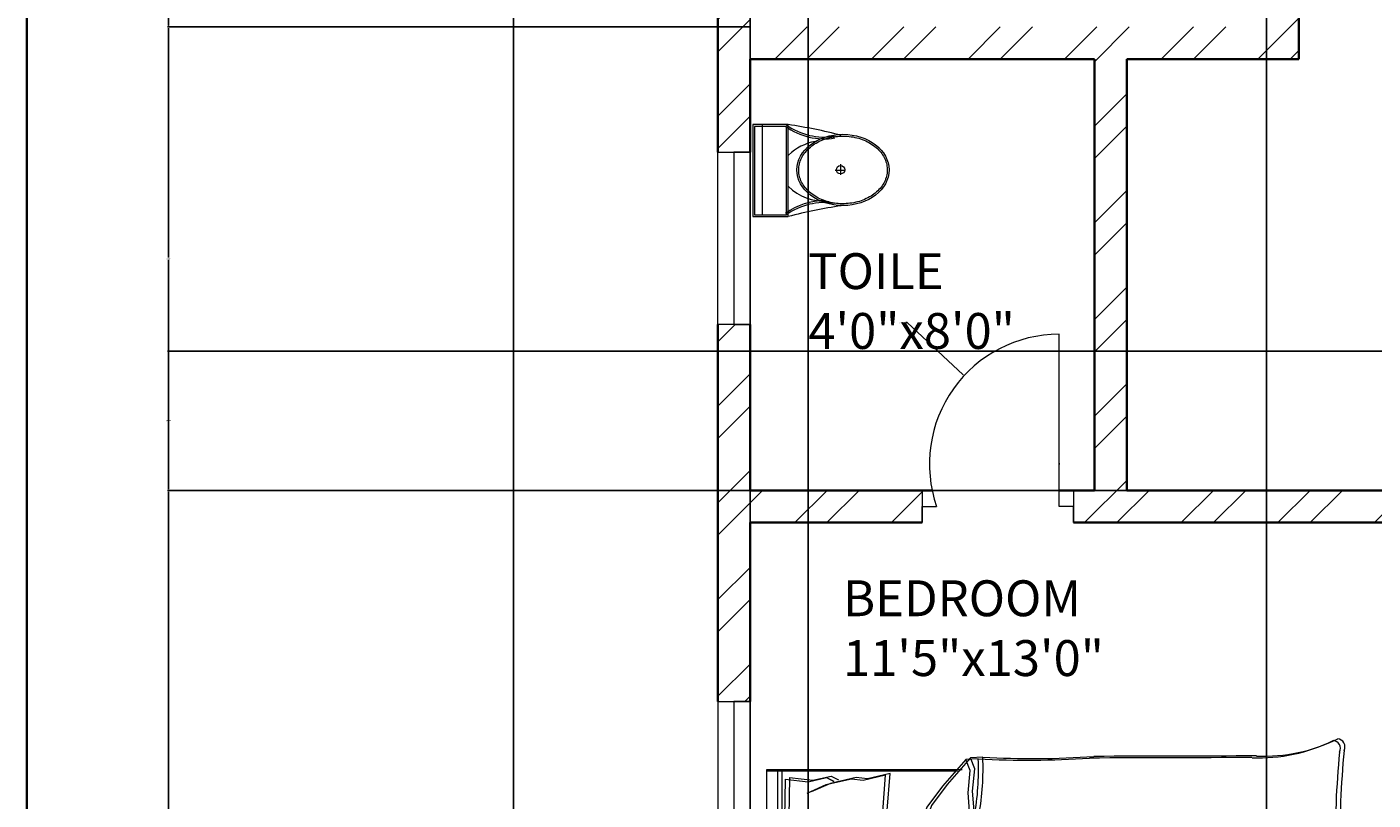
# Model space of a CAD drawing. Units: inches. Extents: x 2008 to 2657, y 1077 to 2165.
# Tile 2 of 16: x 2008 to 2196, y 1309 to 1417. Entities that reach past the tile are written whole.
import ezdxf

# ---------------------------------------------------------------- set-up
doc = ezdxf.new("R2010")
doc.units = ezdxf.units.IN
for name, color, linetype, lineweight in [('A-ANNO-DIMS', 2, 'Continuous', 18), ('A-ANNO-TTLB', 7, 'Continuous', 35), ('A-AREA-IDEN', 4, 'Continuous', 18), ('A-DOOR', 11, 'Continuous', 18), ('A-FLOR-FIXT', 8, 'Continuous', 18), ('A-FURN', 8, 'Continuous', 13), ('A-GLAZ', 191, 'Continuous', 18), ('A-WALL', 7, 'Continuous', 35)]:
    doc.layers.add(name, color=color, linetype=linetype, lineweight=lineweight)
doc.layers.add('A-WALL-PATT', color=30, linetype='Continuous', lineweight=13, true_color=0xf8991e)
doc.styles.get("Standard").update_dxf_attribs({"font": 'arial.ttf'})
doc.dimstyles.get("Standard").update_dxf_attribs({"dimtxt": 0.18, "dimasz": 0.18, "dimexe": 0.18, "dimexo": 0.0625, "dimgap": 0.09, "dimtad": 0, "dimtih": 1, "dimtoh": 1, "dimdec": 4, "dimzin": 0, "dimdsep": 46, "dimtxsty": 'Standard', "dimcen": 0.09, "dimadec": 0, "dimazin": 0, "dimtfac": 1, "dimtdec": 4, "dimtofl": 0, "dimtmove": 0, "dimatfit": 3, "dimfxl": 1, "dimtolj": 1, "dimtzin": 0, "dimarcsym": 0})

# ---------------------------------------------------------------- blocks, each defined once
blk = doc.blocks.new('A$C31115884')
for p, q in [((283.1, 497.7), (223.4, 497.7)), ((257.5, 466.4), (257.5, 523.2)), ((0, 200), (0, 0)), ((520, 200), (0, 200)), ((10, 190), (10, 10)), ((510, 190), (10, 190)), ((510, 10), (510, 190)), ((520, 0), (520, 200)), ((510, 54.5), (0, 54.5)), ((10, 10), (510, 10)), ((0, 0), (520, 0))]:
    blk.add_line(p, q)
blk.add_circle((255.6, 496.4), 23.6)
for centre, radius, start, end in [((2777.7, -204.6), 2807, 165.4549, 171.71327), ((-294.5, 403.3), 364.7, 324.20913, 9.34987), ((-294.5, 403.3), 374.7, 324.20913, 9.34987), ((805.8, 403.3), 364.7, 170.65013, 215.79087), ((3237, 905), 2807, 188.28673, 194.5451), ((139.5, 406.2), 293.5, 315.84364, 2.65635), ((805.8, 403.3), 374.7, 179.20365, 215.79087), ((383.6, 406.2), 293.5, 190.27735, 224.15636)]:
    blk.add_arc(centre, radius, start, end)
blk.add_ellipse((256.2, 509.9), major_axis=(0, -260.7), ratio=0.772727)
blk.add_open_spline([(256.2, 259.2), (263.1, 259.2), (270, 259.7), (287.8, 262.3), (298.7, 265.1), (319.9, 273.1), (330.2, 278.4), (350.1, 291.1), (359.7, 298.7), (377.7, 315.9), (386.2, 325.5), (401.7, 346.6), (408.8, 358.1), (421.3, 382.5), (426.8, 395.5), (435.9, 422.4), (439.5, 436.4), (444.8, 465.1), (446.5, 479.7), (447.9, 509.2), (447.6, 524), (445, 553.3), (442.7, 567.8), (436.3, 596), (432.1, 609.7), (421.9, 636), (416, 648.6), (402.5, 672.1), (395, 683), (378.6, 703), (369.8, 712.1), (351.1, 728), (341.3, 734.8), (320.9, 746.2), (310.4, 750.7), (288.9, 757.3), (278, 759.4), (256, 761), (245, 760.6), (223.1, 757.2), (212.3, 754.3), (191.1, 746.1), (180.8, 740.7), (160.9, 727.8), (151.4, 720.1), (133.5, 702.7), (125.1, 693), (109.6, 671.7), (102.6, 660.2), (90.2, 635.7), (84.9, 622.7), (76, 595.6), (72.4, 581.6), (67.2, 552.9), (65.6, 538.2), (64.4, 508.8), (64.8, 494), (67.5, 464.7), (69.9, 450.2), (76.6, 422), (80.8, 408.3), (91.1, 382.2), (97.2, 369.7), (110.8, 346.3), (118.4, 335.4), (134.8, 315.6), (143.7, 306.7), (162.4, 290.9), (172.3, 284.2), (192.8, 273), (203.3, 268.6), (224.8, 262.2), (235.8, 260.2), (249.9, 259.3), (253, 259.2), (256.2, 259.2)], degree=3, knots=[0, 0, 0, 0, 0.110105, 0.110105, 0.285049, 0.285049, 0.459994, 0.459994, 0.634938, 0.634938, 0.809882, 0.809882, 0.984827, 0.984827, 1.159771, 1.159771, 1.334715, 1.334715, 1.50966, 1.50966, 1.684604, 1.684604, 1.859549, 1.859549, 2.034493, 2.034493, 2.209437, 2.209437, 2.384382, 2.384382, 2.559326, 2.559326, 2.73427, 2.73427, 2.909215, 2.909215, 3.084159, 3.084159, 3.259103, 3.259103, 3.434048, 3.434048, 3.608992, 3.608992, 3.783936, 3.783936, 3.958881, 3.958881, 4.133825, 4.133825, 4.30877, 4.30877, 4.483714, 4.483714, 4.658658, 4.658658, 4.833603, 4.833603, 5.008547, 5.008547, 5.183491, 5.183491, 5.358436, 5.358436, 5.53338, 5.53338, 5.708324, 5.708324, 5.883269, 5.883269, 6.058213, 6.058213, 6.233158, 6.233158, 6.283185, 6.283185, 6.283185, 6.283185])
blk = doc.blocks.new('BED-DOUBLE')
for p, q in [((27.75, 52.87), (24.5, 49.16)), ((27.75, 52.87), (24.5, 49.16)), ((28.39, 53.1), (25.14, 49.39)), ((28.39, 53.1), (25.14, 49.39)), ((29.49, 52.95), (27.75, 52.87, 3.87)), ((29.49, 52.95), (27.75, 52.87, 3.87)), ((28.37, 51.33), (27.75, 52.87)), ((28.37, 51.33), (27.75, 52.87)), ((30.13, 53.18), (28.39, 53.1, 3.87)), ((30.13, 53.18), (28.39, 53.1, 3.87)), ((29, 51.56), (28.39, 53.1)), ((29, 51.56), (28.39, 53.1)), ((0, 51.49), (0.64, 51.49)), ((0, 3.48), (0, 51.49)), ((0, 51.27), (26.61, 51.27)), ((0, 51.27), (26.61, 51.27)), ((0.64, 51.49), (27.25, 51.49)), ((0.64, 51.49), (27.25, 51.49)), ((1.53, 3.48), (1.53, 51.27)), ((1.53, 3.48), (1.53, 51.27)), ((2.17, 3.7), (2.17, 51.49)), ((2.17, 3.7), (2.17, 51.49)), ((16.57, 50.7), (13.43, 49.92)), ((16.57, 50.7), (13.43, 49.92)), ((17.21, 50.93), (14.07, 50.15)), ((17.21, 50.93), (14.07, 50.15)), ((16.17, 45.57), (16.57, 50.7)), ((16.17, 45.57), (16.57, 50.7)), ((16.81, 45.8), (17.21, 50.93)), ((16.81, 45.8), (17.21, 50.93)), ((28.06, 48.23), (28.37, 51.33)), ((28.06, 48.23), (28.37, 51.33)), ((28.7, 48.46), (29, 51.56)), ((28.7, 48.46), (29, 51.56)), ((2.56, 50.11), (2.46, 44.71)), ((2.56, 50.11), (2.46, 44.71)), ((2.56, 50.11), (5.77, 49.73)), ((2.56, 50.11), (5.77, 49.73)), ((3.2, 50.34), (3.1, 44.94)), ((3.2, 50.34), (3.1, 44.94)), ((3.2, 50.34), (6.41, 49.96)), ((3.2, 50.34), (6.41, 49.96)), ((8.26, 49.31), (5.58, 48.13)), ((8.26, 49.31), (5.58, 48.13)), ((5.77, 49.73), (8.34, 50.33)), ((5.77, 49.73), (8.34, 50.33)), ((8.9, 49.54), (6.22, 48.36)), ((8.9, 49.54), (6.22, 48.36)), ((6.41, 49.96), (8.98, 50.56)), ((6.41, 49.96), (8.98, 50.56)), ((11.83, 50.11), (8.26, 49.31)), ((11.83, 50.11), (8.26, 49.31)), ((8.34, 50.33), (9.38, 49.82)), ((8.34, 50.33), (9.38, 49.81)), ((12.47, 50.34), (8.9, 49.54)), ((12.47, 50.34), (8.9, 49.54)), ((8.98, 50.56), (10.02, 50.04)), ((8.98, 50.56), (10.02, 50.04)), ((13.43, 49.92), (11.83, 50.11)), ((13.43, 49.92), (11.83, 50.11)), ((14.07, 50.15), (12.47, 50.34)), ((14.07, 50.15), (12.47, 50.34)), ((24.5, 49.16), (22.33, 46.22)), ((24.5, 49.16), (22.33, 46.22)), ((25.14, 49.39), (22.97, 46.45)), ((25.14, 49.39), (22.97, 46.45)), ((28.37, 44.36), (28.06, 48.23)), ((28.37, 44.36), (28.06, 48.23)), ((29, 44.59), (28.7, 48.46)), ((29, 44.59), (28.7, 48.46)), ((2.46, 44.71), (2.54, 45.71)), ((2.46, 44.71), (2.54, 45.71)), ((2.54, 45.71), (3.07, 41.91)), ((2.54, 45.71), (3.07, 41.91)), ((3.1, 44.94), (3.18, 45.94)), ((3.1, 44.94), (3.18, 45.94)), ((3.18, 45.94), (3.71, 42.14)), ((3.18, 45.94), (3.71, 42.14)), ((16.73, 43.61), (16.17, 45.57)), ((16.73, 43.61), (16.17, 45.57)), ((17.37, 43.84), (16.81, 45.8)), ((17.37, 43.83), (16.81, 45.8)), ((22.33, 46.22), (20.32, 40.64)), ((22.33, 46.22), (20.32, 40.64)), ((22.97, 46.45), (20.96, 40.87)), ((22.97, 46.45), (20.96, 40.87)), ((16.3, 36.6), (16.73, 43.61)), ((16.3, 36.6), (16.73, 43.61)), ((16.93, 36.83), (17.37, 43.84)), ((16.93, 36.82), (17.37, 43.83)), ((28.83, 40.95), (28.37, 44.36)), ((28.83, 40.95), (28.37, 44.36)), ((29.47, 41.18), (29, 44.59)), ((29.47, 41.18), (29, 44.59)), ((3.07, 41.91), (4.42, 36.5)), ((3.07, 41.91), (4.42, 36.5)), ((3.71, 42.14), (5.06, 36.72)), ((3.71, 42.14), (5.06, 36.72)), ((4.31, 39.43), (3.72, 37.36)), ((4.31, 39.43), (3.72, 37.36)), ((20.32, 40.64), (17.38, 32.31)), ((20.32, 40.64), (17.38, 32.31)), ((20.96, 40.87), (18.02, 32.54)), ((20.96, 40.87), (18.02, 32.53)), ((29.76, 38.94), (28.83, 40.95)), ((29.76, 38.94), (28.83, 40.95)), ((30.4, 39.17), (29.47, 41.18)), ((30.4, 39.17), (29.47, 41.18)), ((79.25, 15.06), (79.25, 39.68)), ((79.25, 15.06), (79.25, 39.68)), ((79.88, 15.29), (79.88, 39.91)), ((79.88, 15.29), (79.88, 39.91)), ((3.67, 39.2), (3.08, 37.14)), ((3.67, 39.2), (3.08, 37.14)), ((30.38, 36.46), (29.76, 38.94)), ((30.38, 36.46), (29.76, 38.94)), ((31.02, 36.69), (30.4, 39.17)), ((31.02, 36.69), (30.4, 39.17)), ((3.08, 37.14), (2.54, 34.21)), ((3.08, 37.14), (2.54, 34.2)), ((3.72, 37.36), (3.18, 34.43)), ((3.72, 37.36), (3.18, 34.43)), ((15.63, 32.56), (16.3, 36.6)), ((15.63, 32.56), (16.3, 36.6)), ((16.27, 32.79), (16.93, 36.83)), ((16.27, 32.79), (16.93, 36.82)), ((23.88, 34.45), (28.37, 36.15)), ((23.88, 34.45), (28.37, 36.15)), ((24.52, 34.68), (29, 36.38)), ((24.52, 34.68), (29, 36.38)), ((28.37, 36.15), (30.38, 36.46)), ((28.37, 36.15), (30.38, 36.46)), ((29, 36.38), (31.02, 36.69)), ((29, 36.38), (31.02, 36.69)), ((2.54, 34.21), (2.56, 33.88)), ((2.54, 34.2), (2.56, 33.88)), ((2.56, 33.88), (2.98, 29.46)), ((2.56, 33.88), (2.98, 29.46)), ((3.18, 34.43), (3.2, 34.11)), ((3.18, 34.43), (3.2, 34.11)), ((3.2, 34.11), (3.62, 29.68)), ((3.2, 34.11), (3.62, 29.68)), ((16.74, 30.75), (15.45, 33.82)), ((16.74, 30.75), (15.45, 33.82)), ((17.38, 30.98), (16.09, 34.05)), ((17.38, 30.98), (16.09, 34.05)), ((17.38, 30.26), (23.88, 34.45)), ((17.38, 30.26), (23.88, 34.45)), ((18.02, 30.49), (24.52, 34.68)), ((18.02, 30.49), (24.52, 34.68)), ((16.89, 28.3), (16.74, 30.75)), ((16.89, 28.3), (16.74, 30.75)), ((17.53, 28.53), (17.38, 30.98)), ((17.53, 28.53), (17.38, 30.98)), ((2.98, 29.46), (2.49, 27.98)), ((2.98, 29.46), (2.49, 27.98)), ((3.62, 29.68), (3.13, 28.21)), ((3.62, 29.68), (3.13, 28.21)), ((3.13, 28.21), (8.51, 27.96)), ((3.13, 28.21), (8.51, 27.96)), ((13.02, 27.66), (14.86, 28.36)), ((13.02, 27.66), (14.86, 28.36)), ((14.22, 28.13), (16.89, 28.3)), ((14.22, 28.13), (16.89, 28.3)), ((14.86, 28.36), (17.53, 28.53)), ((14.86, 28.36), (17.53, 28.53)), ((1.87, 25.98), (7.22, 26.56)), ((1.87, 25.98), (7.22, 26.56)), ((2.49, 27.98), (7.87, 27.73)), ((2.49, 27.98), (7.87, 27.73)), ((2.51, 26.21), (7.86, 26.79)), ((2.51, 26.21), (7.86, 26.79)), ((7.22, 26.56), (10.4, 27.14)), ((7.22, 26.56), (10.4, 27.14)), ((7.86, 26.79), (11.04, 27.37)), ((7.86, 26.79), (11.04, 27.37)), ((7.87, 27.73), (11.08, 27.36)), ((7.87, 27.73), (11.08, 27.36)), ((8.51, 27.96), (11.72, 27.58)), ((8.51, 27.96), (11.72, 27.58)), ((10.4, 27.14), (11.7, 27.14)), ((10.4, 27.14), (11.7, 27.14)), ((11.04, 27.37), (12.34, 27.37)), ((11.04, 27.37), (12.34, 27.37)), ((11.08, 27.36), (12.38, 27.44)), ((11.08, 27.36), (12.38, 27.44)), ((11.7, 27.14), (13.58, 26.56)), ((11.7, 27.14), (13.58, 26.56)), ((11.72, 27.58), (13.02, 27.66)), ((11.72, 27.58), (13.02, 27.66)), ((12.34, 27.37), (14.22, 26.79)), ((12.34, 27.37), (14.22, 26.79)), ((12.38, 27.44), (14.22, 28.13)), ((12.38, 27.44), (14.22, 28.13)), ((13.58, 26.56), (16.26, 26.56)), ((13.58, 26.56), (16.26, 26.56)), ((14.22, 26.79), (16.9, 26.79)), ((14.22, 26.79), (16.9, 26.79)), ((16.26, 26.56), (16.26, 24.1)), ((16.26, 26.56), (16.26, 24.1)), ((16.9, 26.79), (16.9, 24.33)), ((16.9, 26.79), (16.9, 24.33)), ((2.45, 24.54), (1.87, 25.98)), ((2.45, 24.54), (1.87, 25.98)), ((2.3, 20.09), (2.45, 24.54)), ((2.3, 20.09), (2.45, 24.54)), ((3.09, 24.77), (2.51, 26.21)), ((3.09, 24.77), (2.51, 26.21)), ((2.94, 20.32), (3.09, 24.77)), ((2.94, 20.32), (3.09, 24.77)), ((16.17, 19.38), (16.57, 24.52)), ((16.17, 19.38), (16.57, 24.52)), ((16.81, 19.61), (17.21, 24.74)), ((16.81, 19.61), (17.21, 24.74)), ((16.26, 24.1), (15.17, 20.96)), ((16.26, 24.1), (15.17, 20.96)), ((16.9, 24.33), (15.81, 21.19)), ((16.9, 24.33), (15.81, 21.19)), ((2.3, 19.77), (2.3, 20.09)), ((2.3, 19.77), (2.3, 20.09)), ((3.03, 16.88), (2.3, 19.77)), ((3.03, 16.88), (2.3, 19.77)), ((2.94, 20), (2.94, 20.32)), ((2.94, 20), (2.94, 20.32)), ((3.67, 17.11), (2.94, 20)), ((3.67, 17.11), (2.94, 20)), ((16.73, 17.42), (16.17, 19.38)), ((16.73, 17.42), (16.17, 19.38)), ((17.37, 17.65), (16.81, 19.61)), ((17.37, 17.65), (16.81, 19.61)), ((3.32, 12.11), (4.33, 17.6)), ((3.32, 12.11), (4.33, 17.6)), ((4.39, 15.08), (3.67, 17.11)), ((4.39, 15.08), (3.67, 17.11)), ((3.96, 12.34), (4.97, 17.83)), ((3.96, 12.34), (4.97, 17.83)), ((16.3, 10.41), (16.73, 17.42)), ((16.3, 10.41), (16.73, 17.42)), ((16.93, 10.64), (17.37, 17.65)), ((16.93, 10.64), (17.37, 17.65)), ((3.75, 14.86), (3.03, 16.88)), ((3.75, 14.86), (3.03, 16.88)), ((3.03, 8.29), (3.32, 12.11)), ((3.03, 8.29), (3.32, 12.11)), ((3.67, 8.51), (3.96, 12.34)), ((3.67, 8.51), (3.96, 12.34)), ((15.63, 6.38), (16.3, 10.41)), ((15.63, 6.38), (16.3, 10.41)), ((16.27, 6.61), (16.93, 10.64)), ((16.27, 6.61), (16.93, 10.64)), ((16.3, 10.41), (16.62, 9.28)), ((16.3, 10.41), (16.62, 9.28)), ((16.93, 10.64), (17.26, 9.51)), ((16.93, 10.64), (17.26, 9.51)), ((17.26, 9.51), (17.98, 4.41)), ((17.26, 9.51), (17.98, 4.41)), ((3.01, 8.18), (3.03, 8.29)), ((3.01, 8.18), (3.03, 8.29)), ((3.34, 3.9), (3.01, 8.18)), ((3.34, 3.9), (3.01, 8.18)), ((3.65, 8.41), (3.67, 8.51)), ((3.65, 8.41), (3.67, 8.51)), ((3.98, 4.13), (3.65, 8.41)), ((3.98, 4.13), (3.65, 8.41)), ((16.62, 9.28), (17.34, 4.18)), ((16.62, 9.28), (17.34, 4.18)), ((8.96, 5.05), (6.21, 6.06)), ((8.96, 5.05), (6.21, 6.06)), ((9.59, 5.28), (6.85, 6.29)), ((9.59, 5.28), (6.85, 6.29)), ((3.32, 3.9), (6.5, 4.47)), ((3.32, 3.89), (6.5, 4.47)), ((3.96, 4.12), (7.14, 4.7)), ((3.96, 4.12), (7.14, 4.7)), ((6.5, 4.47), (9.1, 4.04)), ((6.5, 4.47), (9.1, 4.04)), ((7.14, 4.7), (9.74, 4.27)), ((7.14, 4.7), (9.74, 4.27)), ((12.57, 4.47), (8.96, 5.05)), ((12.57, 4.47), (8.96, 5.05)), ((9.1, 4.04), (10.11, 4.62)), ((9.1, 4.04), (10.11, 4.62)), ((13.21, 4.7), (9.59, 5.28)), ((13.21, 4.7), (9.59, 5.28)), ((9.74, 4.27), (10.75, 4.85)), ((9.74, 4.27), (10.75, 4.85)), ((14.16, 4.76), (12.57, 4.47)), ((14.16, 4.76), (12.57, 4.47)), ((14.8, 4.99), (13.21, 4.7)), ((14.8, 4.99), (13.21, 4.7)), ((17.34, 4.18), (14.16, 4.76)), ((17.34, 4.18), (14.16, 4.76)), ((17.98, 4.41), (14.8, 4.99)), ((17.98, 4.41), (14.8, 4.99)), ((18.11, 3.48), (0, 3.48)), ((18.11, 3.48), (0, 3.48)), ((18.75, 3.7), (0.64, 3.7)), ((18.75, 3.7), (0.64, 3.7))]:
    blk.add_line(p, q)
for centre, radius, start, end in [((68.67, 76.16), 23.07, 267.4714, 296.4681), ((68.67, 76.16), 23.07, 267.4714, 296.4681), ((69.31, 76.39), 23.07, 267.4714, 296.4681), ((69.31, 76.39), 23.07, 267.4714, 296.4681), ((78.87, 54.41), 1.1, 332.6588, 86.02), ((78.87, 54.41), 1.1, 332.6588, 86.02), ((79.51, 54.64), 1.1, 332.6588, 86.02), ((79.51, 54.64), 1.1, 332.6588, 86.02), ((-6.66, 51.33), 36.18, 349.8763, 2.5657), ((-6.66, 51.33), 36.18, 349.8763, 2.5657), ((36.32, 182.27), 129.5, 266.9791, 273.8365), ((36.32, 182.27), 129.5, 266.9791, 273.8365), ((-6.02, 51.56), 36.18, 349.8763, 2.5657), ((-6.02, 51.56), 36.18, 349.8763, 2.5657), ((36.95, 182.49), 129.5, 266.9791, 273.8365), ((36.95, 182.49), 129.5, 266.9791, 273.8365), ((67.82, -4508.74), 4561.86, 90.00217, 90.28689), ((67.82, -4508.74), 4561.86, 90.00217, 90.28689), ((68.46, -4508.51), 4561.86, 90.00217, 90.28689), ((68.46, -4508.51), 4561.86, 90.00217, 90.28689), ((212.28, 41.15), 133.04, 174.4998, 180.6351), ((212.28, 41.15), 133.04, 174.4998, 180.6351), ((212.92, 41.38), 133.04, 174.4998, 180.6351), ((212.92, 41.38), 133.04, 174.4998, 180.6351), ((35.71, 43.97), 6.22, 168.6608, 203.7384), ((35.71, 43.97), 6.22, 168.6608, 203.7384), ((35.07, 43.74), 6.22, 168.6608, 203.7384), ((35.07, 43.74), 6.22, 168.6608, 203.7384), ((2.12, 31.38), 29.65, 10.6617, 19.8806), ((2.12, 31.38), 29.65, 10.6617, 19.8806), ((1.48, 31.15), 29.65, 10.6617, 19.8806), ((1.48, 31.15), 29.65, 10.6617, 19.8806), ((156.32, 17.76), 129.02, 171.7845, 186.9006), ((156.32, 17.76), 129.02, 171.7845, 186.9006), ((156.96, 17.98), 129.02, 171.7845, 186.9006), ((156.96, 17.98), 129.02, 171.7845, 186.9006), ((30.44, 36.64), 0.185, 250.2464, 1.1377), ((30.44, 36.64), 0.185, 250.2464, 1.1377), ((31.08, 36.87), 0.185, 250.2464, 1.1377), ((31.08, 36.86), 0.185, 250.2464, 1.1377), ((182.05, 21.36), 164.97, 176.0865, 186.7821), ((182.05, 21.36), 164.97, 176.0865, 186.7821), ((182.69, 21.59), 164.97, 176.0865, 186.7821), ((182.69, 21.59), 164.97, 176.0865, 186.7821), ((-23.71, -17.22), 106.46, 13.3832, 17.7053), ((-23.71, -17.22), 106.46, 13.3832, 17.7053), ((-23.07, -16.99), 106.46, 13.3832, 17.7053), ((-23.07, -16.99), 106.46, 13.3832, 17.7053), ((200.84, 21.43), 121.76, 182.9958, 189.4091), ((200.84, 21.43), 121.76, 182.9958, 189.4091), ((201.48, 21.66), 121.76, 182.9958, 189.4091), ((201.48, 21.66), 121.76, 182.9958, 189.4091), ((20.1, 85.16), 83.31, 268.7218, 275.604), ((20.1, 85.16), 83.31, 268.7218, 275.604), ((20.74, 85.39), 83.31, 268.7218, 275.604), ((20.74, 85.39), 83.31, 268.7218, 275.604), ((31.17, -167.31), 170.11, 88.4762, 91.0082), ((31.17, -167.31), 170.11, 88.4762, 91.0082), ((31.81, -167.08), 170.11, 88.4762, 91.0082), ((31.81, -167.08), 170.11, 88.4762, 91.0082), ((50.61, 484.82), 482.31, 268.2277, 271.7185), ((50.61, 484.82), 482.31, 268.2277, 271.7185), ((51.25, 485.05), 482.31, 268.2277, 271.7185), ((51.25, 485.05), 482.31, 268.2277, 271.7185), ((64.52, -26.9), 29.63, 76.0648, 88.9113), ((64.52, -26.9), 29.63, 76.0648, 88.9113), ((65.15, -26.67), 29.63, 76.0648, 88.9113), ((65.15, -26.67), 29.63, 76.0648, 88.9113), ((70.92, -21.43), 23.56, 67.9751, 86.652), ((70.92, -21.43), 23.56, 67.9751, 86.652), ((70.28, -21.66), 23.56, 67.9751, 86.652), ((70.28, -21.66), 23.56, 67.9751, 86.652), ((79.72, 1.09), 1.09, 236.1736, 23.4781), ((79.72, 1.09), 1.09, 236.1736, 23.4781), ((80.36, 1.32), 1.09, 236.1736, 23.4781), ((80.36, 1.32), 1.09, 236.1736, 23.4781)]:
    blk.add_arc(centre, radius, start, end)
blk = doc.blocks.new('WIN-24IN-A')
for p, q in [((0, 24), (4.5, 24)), ((0, 0), (0, 24)), ((4.5, 24), (2.25, 24)), ((2.25, 24), (2.25, 0)), ((4.5, 24), (4.5, 0)), ((4.5, 0), (0, 0)), ((2.25, 0), (4.5, 0))]:
    blk.add_line(p, q)
blk = doc.blocks.new('WIN-60IN-A')
for p, q in [((0, 60), (4.5, 60)), ((0, 60), (0, 0)), ((4.5, 60), (2.25, 60)), ((2.25, 60), (2.25, 0)), ((4.5, 0), (4.5, 60)), ((4.5, 0), (0, 0)), ((2.25, 0), (4.5, 0))]:
    blk.add_line(p, q)
blk = doc.blocks.new('*D31')
at = {"layer": 'A-ANNO-DIMS', "color": 0, "lineweight": -2, "transparency": 16777216}
for p, q in [((2076.26, 1562.18), (2076.26, 1140.44)), ((2576.76, 1188.61), (2576.76, 1140.44)), ((2076.44, 1140.62), (2326.12, 1140.62)), ((2576.58, 1140.62), (2326.91, 1140.62))]:
    blk.add_line(p, q, dxfattribs=at)
at = {"layer": 'A-ANNO-DIMS', "color": 0, "transparency": 16777216}
for points in [[(2076.44, 1140.65), (2076.44, 1140.59), (2076.26, 1140.62)], [(2576.58, 1140.65), (2576.58, 1140.59), (2576.76, 1140.62)]]:
    blk.add_solid(points, dxfattribs=at)
at = {"layer": 'Defpoints', "color": 0, "transparency": 16777216}
for p in [(2076.26, 1562.24), (2576.76, 1188.67), (2576.76, 1140.62)]:
    blk.add_point(p, dxfattribs=at)
at = {"layer": 'A-ANNO-DIMS', "color": 0, "transparency": 16777216, "insert": (2326.51, 1140.62), "char_height": 0.18, "attachment_point": 5}
blk.add_mtext('\\A1;500.5', dxfattribs=at)
blk = doc.blocks.new('*D39')
at = {"layer": 'A-ANNO-DIMS', "color": 0, "lineweight": -2, "transparency": 16777216}
for p, q in [((2109.2, 1352.17), (2028.03, 1352.17)), ((2028.21, 1351.99), (2028.21, 1290.11)), ((2028.21, 1227.85), (2028.21, 1289.74)), ((2109.2, 1227.67), (2028.03, 1227.67))]:
    blk.add_line(p, q, dxfattribs=at)
at = {"layer": 'A-ANNO-DIMS', "color": 0, "transparency": 16777216}
for points in [[(2028.18, 1351.99), (2028.24, 1351.99), (2028.21, 1352.17)], [(2028.18, 1227.85), (2028.24, 1227.85), (2028.21, 1227.67)]]:
    blk.add_solid(points, dxfattribs=at)
at = {"layer": 'Defpoints', "color": 0, "transparency": 16777216}
for p in [(2028.21, 1352.17), (2109.26, 1352.17), (2109.26, 1227.67)]:
    blk.add_point(p, dxfattribs=at)
at = {"layer": 'A-ANNO-DIMS', "color": 0, "transparency": 16777216, "insert": (2028.21, 1289.92), "char_height": 0.18, "attachment_point": 5}
blk.add_mtext('\\A1;124.5', dxfattribs=at)
blk = doc.blocks.new('*D40')
at = {"layer": 'A-ANNO-DIMS', "color": 0, "lineweight": -2, "transparency": 16777216}
for p, q in [((2109.2, 1416.74), (2028.03, 1416.74)), ((2028.21, 1416.56), (2028.21, 1384.64)), ((2028.21, 1352.35), (2028.21, 1384.28)), ((2109.2, 1352.17), (2028.03, 1352.17))]:
    blk.add_line(p, q, dxfattribs=at)
at = {"layer": 'A-ANNO-DIMS', "color": 0, "transparency": 16777216}
for points in [[(2028.18, 1416.56), (2028.24, 1416.56), (2028.21, 1416.74)], [(2028.18, 1352.35), (2028.24, 1352.35), (2028.21, 1352.17)]]:
    blk.add_solid(points, dxfattribs=at)
at = {"layer": 'Defpoints', "color": 0, "transparency": 16777216}
for p in [(2028.21, 1416.74), (2109.26, 1416.74), (2109.26, 1352.17)]:
    blk.add_point(p, dxfattribs=at)
at = {"layer": 'A-ANNO-DIMS', "color": 0, "transparency": 16777216, "insert": (2028.21, 1384.46), "char_height": 0.18, "attachment_point": 5}
blk.add_mtext('\\A1;64.57', dxfattribs=at)
blk = doc.blocks.new('*D41')
at = {"layer": 'A-ANNO-DIMS', "color": 0, "lineweight": -2, "transparency": 16777216}
for p, q in [((2109.2, 1514.24), (2028.03, 1514.24)), ((2028.21, 1514.06), (2028.21, 1465.67)), ((2028.21, 1416.92), (2028.21, 1465.31)), ((2109.2, 1416.74), (2028.03, 1416.74))]:
    blk.add_line(p, q, dxfattribs=at)
at = {"layer": 'A-ANNO-DIMS', "color": 0, "transparency": 16777216}
for points in [[(2028.18, 1514.06), (2028.24, 1514.06), (2028.21, 1514.24)], [(2028.18, 1416.92), (2028.24, 1416.92), (2028.21, 1416.74)]]:
    blk.add_solid(points, dxfattribs=at)
at = {"layer": 'Defpoints', "color": 0, "transparency": 16777216}
for p in [(2028.21, 1514.24), (2109.26, 1514.24), (2109.26, 1416.74)]:
    blk.add_point(p, dxfattribs=at)
at = {"layer": 'A-ANNO-DIMS', "color": 0, "transparency": 16777216, "insert": (2028.21, 1465.49), "char_height": 0.18, "attachment_point": 5}
blk.add_mtext('\\A1;97.5', dxfattribs=at)
blk = doc.blocks.new('*D55')
at = {"layer": 'A-ANNO-DIMS', "color": 0, "lineweight": -2, "transparency": 16777216}
for p, q in [((2109.26, 1509.68), (2109.26, 1140.44)), ((2181.26, 1509.68), (2181.26, 1140.44)), ((2109.44, 1140.62), (2145.04, 1140.62)), ((2181.08, 1140.62), (2145.48, 1140.62))]:
    blk.add_line(p, q, dxfattribs=at)
at = {"layer": 'A-ANNO-DIMS', "color": 0, "transparency": 16777216}
for points in [[(2109.44, 1140.65), (2109.44, 1140.59), (2109.26, 1140.62)], [(2181.08, 1140.65), (2181.08, 1140.59), (2181.26, 1140.62)]]:
    blk.add_solid(points, dxfattribs=at)
at = {"layer": 'Defpoints', "color": 0, "transparency": 16777216}
for p in [(2109.26, 1509.74), (2181.26, 1509.74), (2109.26, 1140.62)]:
    blk.add_point(p, dxfattribs=at)
at = {"layer": 'A-ANNO-DIMS', "color": 0, "transparency": 16777216, "insert": (2145.26, 1140.62), "char_height": 0.18, "attachment_point": 5}
blk.add_mtext('\\A1;72', dxfattribs=at)
blk = doc.blocks.new('*D62')
at = {"layer": 'A-ANNO-DIMS', "color": 0, "lineweight": -2, "transparency": 16777216}
for p, q in [((2117.38, 1566.68), (2117.38, 1140.44)), ((2237.38, 1566.68), (2237.38, 1140.44)), ((2117.56, 1140.62), (2177.1, 1140.62)), ((2237.2, 1140.62), (2177.66, 1140.62))]:
    blk.add_line(p, q, dxfattribs=at)
at = {"layer": 'A-ANNO-DIMS', "color": 0, "transparency": 16777216}
for points in [[(2117.56, 1140.65), (2117.56, 1140.59), (2117.38, 1140.62)], [(2237.2, 1140.65), (2237.2, 1140.59), (2237.38, 1140.62)]]:
    blk.add_solid(points, dxfattribs=at)
at = {"layer": 'Defpoints', "color": 0, "transparency": 16777216}
for p in [(2117.38, 1566.74), (2237.38, 1566.74), (2237.38, 1140.62)]:
    blk.add_point(p, dxfattribs=at)
at = {"layer": 'A-ANNO-DIMS', "color": 0, "transparency": 16777216, "insert": (2177.38, 1140.62), "char_height": 0.18, "attachment_point": 5}
blk.add_mtext('\\A1;120', dxfattribs=at)
blk = doc.blocks.new('*D68')
at = {"layer": 'A-ANNO-DIMS', "color": 0, "lineweight": -2, "transparency": 16777216}
for p, q in [((2572.2, 1371.57), (2028.03, 1371.57)), ((2028.21, 1371.39), (2028.21, 1362.05)), ((2028.21, 1352.35), (2028.21, 1361.69)), ((2572.2, 1352.17), (2028.03, 1352.17))]:
    blk.add_line(p, q, dxfattribs=at)
at = {"layer": 'A-ANNO-DIMS', "color": 0, "transparency": 16777216}
for points in [[(2028.18, 1371.39), (2028.24, 1371.39), (2028.21, 1371.57)], [(2028.18, 1352.35), (2028.24, 1352.35), (2028.21, 1352.17)]]:
    blk.add_solid(points, dxfattribs=at)
at = {"layer": 'Defpoints', "color": 0, "transparency": 16777216}
for p in [(2028.21, 1371.57), (2572.26, 1371.57), (2572.26, 1352.17)]:
    blk.add_point(p, dxfattribs=at)
at = {"layer": 'A-ANNO-DIMS', "color": 0, "transparency": 16777216, "insert": (2028.21, 1361.87), "char_height": 0.18, "attachment_point": 5}
blk.add_mtext('\\A1;19.394', dxfattribs=at)
blk = doc.blocks.new('*D93')
at = {"layer": 'A-ANNO-DIMS', "color": 0, "lineweight": -2, "transparency": 16777216}
for p, q in [((2130.98, 1375.54), (2131.16, 1375.54)), ((2131.16, 1375.54), (2138.97, 1368.28)), ((2152.25, 1355.85), (2152.43, 1355.85)), ((2152.34, 1355.76), (2152.34, 1355.94))]:
    blk.add_line(p, q, dxfattribs=at)
at = {"layer": 'A-ANNO-DIMS', "color": 0, "transparency": 16777216}
blk.add_solid([(2138.99, 1368.3), (2138.95, 1368.26), (2139.1, 1368.16)], dxfattribs=at)
at = {"layer": 'Defpoints', "color": 0, "transparency": 16777216}
for p in [(2139.1, 1368.16), (2152.34, 1355.85)]:
    blk.add_point(p, dxfattribs=at)
at = {"layer": 'A-ANNO-DIMS', "color": 0, "transparency": 16777216, "insert": (2130.43, 1375.54), "char_height": 0.18, "attachment_point": 5}
blk.add_mtext('\\A1;R18.075', dxfattribs=at)

msp = doc.modelspace()

# ---------------------------------------------------------------- hatches: boundary and pattern name
at = {"layer": 'A-WALL-PATT'}
h = msp.add_hatch(dxfattribs=at)
h.set_pattern_fill('ANSI32', color=256)
h.paths.add_polyline_path([(2109.2619, 2094.6743), (2104.7619, 2094.6743), (2104.7619, 2072.1743), (2104.7619, 2021.6151), (2109.2619, 2021.6151), (2109.2619, 2055.6743), (2126.1387, 2055.6743), (2126.1387, 2057.9243), (2126.1387, 2060.1743), (2109.2619, 2060.1743)])
h.paths.add_polyline_path([(2223.2494, 2057.9243), (2223.2494, 2060.1743), (2186.1387, 2060.1743), (2186.1387, 2055.6743), (2223.2494, 2055.6743)])
h.paths.add_polyline_path([(2250.7619, 2072.1743), (2250.7619, 2090.1743), (2250.7619, 2094.6743), (2246.2619, 2094.6743), (2246.2619, 2060.1743), (2242.7242, 2060.1743), (2242.7242, 2055.6743), (2246.2619, 2055.6743), (2246.2619, 1899.6743), (2242.7458, 1899.6743), (2242.7458, 1897.4243), (2242.7458, 1895.1743), (2246.2619, 1895.1743), (2246.2619, 1878.8745), (2248.5119, 1878.8745), (2250.7619, 1878.8745), (2250.7619, 1991.1743), (2250.7619, 2025.6743), (2257.6798, 2025.6743), (2257.6798, 2027.9243), (2257.6798, 2030.1743), (2250.7619, 2030.1743)])
h.paths.add_polyline_path([(2411.2619, 2031.6743), (2409.0119, 2031.6743), (2406.7619, 2031.6743), (2406.7619, 2030.1743), (2322.7619, 2030.1743), (2322.7619, 2053.3443), (2318.2619, 2053.3443), (2318.2619, 2030.1743), (2305.6798, 2030.1743), (2305.6798, 2025.6743), (2318.2619, 2025.6743), (2322.7619, 2025.6743), (2406.7619, 2025.6743), (2406.7619, 1995.6743), (2406.7619, 1847.2677), (2250.7619, 1847.2677), (2250.7619, 1850.9902), (2248.5119, 1850.9902), (2246.2619, 1850.9902), (2246.2619, 1847.1743), (2246.2619, 1842.7677), (2303.0015, 1842.7677), (2303.0015, 1667.2413), (2298.4208, 1667.2413), (2298.4208, 1662.7413), (2303.0015, 1662.7413), (2303.0015, 1649.8758), (2307.5015, 1649.8758), (2307.5015, 1842.7677), (2406.7619, 1842.7677), (2411.2619, 1842.7677), (2411.2619, 1878.6743), (2415.8196, 1878.6743), (2415.8196, 1880.9243), (2415.8196, 1883.1743), (2411.2619, 1883.1743)])
h.paths.add_polyline_path([(2411.2619, 2094.6743), (2406.7619, 2094.6743), (2318.2619, 2094.6743), (2318.2619, 2077.3443), (2322.7619, 2077.3443), (2322.7619, 2090.1743), (2406.7619, 2090.1743), (2406.7619, 2072.1743), (2406.7619, 2067.6743), (2406.7619, 2052.7524), (2411.2619, 2052.7524), (2411.2619, 2055.6743), (2414.9888, 2055.6743), (2414.9888, 2057.9243), (2414.9888, 2060.1743), (2411.2619, 2060.1743), (2411.2619, 2072.1743)])
h.paths.add_polyline_path([(2576.7619, 2072.1743), (2576.7619, 2094.6743), (2572.2619, 2094.6743), (2572.2619, 2060.1743), (2525.8113, 2060.1743), (2525.8113, 2055.6743), (2572.2619, 2055.6743), (2572.2619, 1994.289), (2576.7619, 1994.289)])
h.paths.add_polyline_path([(2465.8113, 2060.1743), (2436.2802, 2060.1743), (2436.2802, 2055.6743), (2465.8113, 2055.6743), (2465.8113, 2057.9243)])
h.paths.add_polyline_path([(2576.7619, 1934.289), (2574.5119, 1934.289), (2572.2619, 1934.289), (2572.2619, 1883.1743), (2447.7027, 1883.1743), (2447.7027, 1878.6743), (2459.7619, 1878.6743), (2459.7619, 1830.4982), (2464.2619, 1830.4982), (2464.2619, 1878.6743), (2572.2619, 1878.6743), (2572.2619, 1868.4883), (2576.7619, 1868.4883)])
h.paths.add_polyline_path([(2576.7619, 1832.4883), (2572.2619, 1832.4883), (2572.2619, 1806.6743), (2464.2619, 1806.6743), (2464.2619, 1809.6629), (2459.7619, 1809.6629), (2459.7619, 1802.1743), (2483.7619, 1802.1743), (2483.7619, 1778.1743), (2488.2619, 1778.1743), (2488.2619, 1802.1743), (2572.2619, 1802.1743), (2572.2619, 1793.6101), (2576.7619, 1793.6101)])
h.paths.add_polyline_path([(2576.7619, 1769.6101), (2572.2619, 1769.6101), (2572.2619, 1754.1743), (2488.2619, 1754.1743), (2488.2619, 1757.2675), (2486.0119, 1757.2675), (2483.7619, 1757.2675), (2483.7619, 1754.1743), (2447.4528, 1754.1743), (2447.4528, 1749.6743), (2483.7619, 1749.6743), (2572.2619, 1749.6743), (2572.2619, 1715.1837), (2576.7619, 1715.1837)])
h.paths.add_polyline_path([(2576.7619, 1655.1837), (2572.2619, 1655.1837), (2572.2619, 1617.6743), (2411.2619, 1617.6743), (2411.2619, 1749.6743), (2414.2827, 1749.6743), (2414.2827, 1754.1743), (2406.7619, 1754.1743), (2406.7619, 1749.6743), (2406.7619, 1617.6743), (2307.5015, 1617.6743), (2307.5015, 1621.0007), (2305.2515, 1621.0007), (2303.0015, 1621.0007), (2303.0015, 1609.6944), (2307.5015, 1609.6944), (2307.5015, 1613.1743), (2406.7619, 1613.1743), (2406.7619, 1476.6743), (2415.532, 1476.6743), (2415.532, 1478.9243), (2415.532, 1481.1743), (2411.2619, 1481.1743), (2411.2619, 1613.1743), (2572.2619, 1613.1743), (2572.2619, 1584.6086), (2576.7619, 1584.6086)])
h.paths.add_polyline_path([(2576.7619, 1524.6086), (2572.2619, 1524.6086), (2572.2619, 1481.1743), (2483.7619, 1481.1743), (2447.5119, 1481.1743), (2447.5119, 1476.6743), (2483.7619, 1476.6743), (2483.7619, 1473.5051), (2488.2619, 1473.5051), (2488.2619, 1476.6743), (2572.2619, 1476.6743), (2572.2619, 1469.5488), (2576.7619, 1469.5488)])
h.paths.add_polyline_path([(2576.7619, 1445.5488), (2572.2619, 1445.5488), (2572.2619, 1428.6743), (2488.2619, 1428.6743), (2488.2619, 1455.6743), (2486.0119, 1455.6743), (2483.7619, 1455.6743), (2483.7619, 1428.6743), (2459.7619, 1428.6743), (2459.7619, 1422.1519), (2464.2619, 1422.1519), (2464.2619, 1424.1743), (2572.2619, 1424.1743), (2572.2619, 1407.5685), (2576.7619, 1407.5685)])
h.paths.add_polyline_path([(2576.7619, 1371.5685), (2572.2619, 1371.5685), (2572.2619, 1352.1743), (2464.2619, 1352.1743), (2464.2619, 1403.1384), (2462.0119, 1403.1384), (2459.7619, 1403.1384), (2459.7619, 1352.1743), (2446.3194, 1352.1743), (2446.3194, 1347.6743), (2572.2619, 1347.6743), (2572.2619, 1321.0291), (2576.7619, 1321.0291)])
h.paths.add_polyline_path([(2462.703, 1227.6743), (2436.0298, 1227.6743), (2436.0298, 1225.4243), (2436.0298, 1223.1743), (2462.703, 1223.1743), (2462.703, 1225.4243)])
h.paths.add_polyline_path([(2576.7619, 1261.0291), (2574.5119, 1261.0291), (2572.2619, 1261.0291), (2572.2619, 1227.6743), (2522.703, 1227.6743), (2522.703, 1223.1743), (2572.2619, 1223.1743), (2572.2619, 1188.6743), (2576.7619, 1188.6743), (2576.7619, 1193.1743), (2576.7619, 1223.1743)])
h.paths.add_polyline_path([(2414.2823, 1227.6743), (2411.2619, 1227.6743), (2411.2619, 1267.1779), (2409.0119, 1267.1779), (2406.7619, 1267.1779), (2406.7619, 1227.6743), (2322.7619, 1227.6743), (2322.7619, 1244.3623), (2318.2619, 1244.3623), (2318.2619, 1223.1743), (2406.7619, 1223.1743), (2406.7619, 1193.1743), (2406.7619, 1188.6743), (2411.2619, 1188.6743), (2411.2619, 1193.1743), (2411.2619, 1223.1743), (2414.2823, 1223.1743)])
h.paths.add_polyline_path([(2411.2619, 1347.6743), (2414.702, 1347.6743), (2414.702, 1349.9243), (2414.702, 1352.1743), (2411.2619, 1352.1743), (2411.2619, 1416.7413), (2307.5015, 1416.7413), (2307.5015, 1579.8489), (2305.2515, 1579.8489), (2303.0015, 1579.8489), (2303.0015, 1566.7413), (2299.2719, 1566.7413), (2299.2719, 1562.2413), (2303.0015, 1562.2413), (2303.0015, 1416.7413), (2246.2619, 1416.7413), (2246.2619, 1409.8616), (2250.7619, 1409.8616), (2250.7619, 1412.2413), (2406.7619, 1412.2413), (2406.7619, 1292.1743), (2304.9703, 1292.1743), (2304.9703, 1287.6743), (2318.2619, 1287.6743), (2318.2619, 1268.3623), (2322.7619, 1268.3623), (2322.7619, 1287.6743), (2406.7619, 1287.6743), (2406.7619, 1285.4748), (2411.2619, 1285.4748)])
h.paths.add_polyline_path([(2109.2619, 1262.7482), (2104.7619, 1262.7482), (2104.7619, 1223.1743), (2104.7619, 1193.1743), (2104.7619, 1188.6743), (2109.2619, 1188.6743), (2109.2619, 1223.1743), (2126.7928, 1223.1743), (2126.7928, 1225.4243), (2126.7928, 1227.6743), (2109.2619, 1227.6743)])
h.paths.add_polyline_path([(2222.3268, 1227.6743), (2186.7928, 1227.6743), (2186.7928, 1223.1743), (2222.3268, 1223.1743)])
h.paths.add_polyline_path([(2250.7619, 1287.6743), (2256.9703, 1287.6743), (2256.9703, 1289.9243), (2256.9703, 1292.1743), (2250.7619, 1292.1743), (2250.7619, 1382.2078), (2248.5119, 1382.2078), (2246.2619, 1382.2078), (2246.2619, 1347.6743), (2246.2619, 1227.6743), (2242.6068, 1227.6743), (2242.6068, 1223.1743), (2246.2619, 1223.1743), (2246.2619, 1188.6743), (2250.7619, 1188.6743), (2250.7619, 1193.1743), (2250.7619, 1227.6743)])
h.paths.add_polyline_path([(2133.2619, 1349.9243), (2133.2619, 1352.1743), (2109.2619, 1352.1743), (2109.2619, 1375.2826), (2104.7619, 1375.2826), (2104.7619, 1322.7482), (2109.2619, 1322.7482), (2109.2619, 1347.6743), (2133.2619, 1347.6743)])
h.paths.add_polyline_path([(2210.2105, 1352.1743), (2161.7619, 1352.1743), (2161.7619, 1412.2413), (2185.7619, 1412.2413), (2185.7619, 1420.1851), (2183.5119, 1420.1851), (2181.2619, 1420.1851), (2181.2619, 1416.7413), (2109.2619, 1416.7413), (2109.2619, 1452.4006), (2104.7619, 1452.4006), (2104.7619, 1399.2826), (2109.2619, 1399.2826), (2109.2619, 1412.2413), (2157.2619, 1412.2413), (2157.2619, 1352.1743), (2154.3383, 1352.1743), (2154.3383, 1347.6743), (2210.2105, 1347.6743)])
h.paths.add_polyline_path([(2185.7619, 1514.2413), (2161.7619, 1514.2413), (2161.7619, 1518.1307), (2159.5119, 1518.1307), (2157.2619, 1518.1307), (2157.2619, 1514.2413), (2109.2619, 1514.2413), (2109.2619, 1528.997), (2107.0119, 1528.997), (2104.7619, 1528.997), (2104.7619, 1488.4006), (2109.2619, 1488.4006), (2109.2619, 1509.7413), (2181.2619, 1509.7413), (2181.2619, 1441.2042), (2185.7619, 1441.2042)])
h.paths.add_polyline_path([(2270.4025, 1566.7413), (2109.2619, 1566.7413), (2080.7619, 1566.7413), (2080.7619, 1586.5643), (2076.2619, 1586.5643), (2076.2619, 1562.2413), (2080.7619, 1562.2413), (2104.7619, 1562.2413), (2104.7619, 1552.997), (2109.2619, 1552.997), (2109.2619, 1562.2413), (2157.2619, 1562.2413), (2157.2619, 1538.2413), (2161.7619, 1538.2413), (2161.7619, 1562.2413), (2205.2619, 1562.2413), (2270.4025, 1562.2413)])
h.paths.add_polyline_path([(2131.6813, 1897.4243), (2131.6813, 1899.6743), (2109.2619, 1899.6743), (2109.2619, 1961.6151), (2104.7619, 1961.6151), (2104.7619, 1886.8042), (2109.2619, 1886.8042), (2109.2619, 1895.1743), (2131.6813, 1895.1743)])
h.paths.add_polyline_path([(2185.7619, 1847.1743), (2161.7619, 1847.1743), (2161.7619, 1895.1743), (2185.7619, 1895.1743), (2211.543, 1895.1743), (2211.543, 1897.4243), (2211.543, 1899.6743), (2154.0916, 1899.6743), (2154.0916, 1897.4243), (2154.0916, 1895.1743), (2157.2619, 1895.1743), (2157.2619, 1847.1743), (2109.2619, 1847.1743), (2109.2619, 1862.8042), (2104.7619, 1862.8042), (2104.7619, 1821.243), (2109.2619, 1821.243), (2109.2619, 1842.6743), (2181.2619, 1842.6743), (2181.2619, 1840.6763), (2185.7619, 1840.6763)])
h.paths.add_polyline_path([(2109.2619, 1785.243), (2104.7619, 1785.243), (2104.7619, 1715.4691), (2109.2619, 1715.4691), (2109.2619, 1730.8423), (2157.2619, 1730.8423), (2157.2619, 1727.6404), (2161.7619, 1727.6404), (2161.7619, 1730.8423), (2185.7619, 1730.8423), (2185.7619, 1822.1438), (2183.5119, 1822.1438), (2181.2619, 1822.1438), (2181.2619, 1735.3423), (2109.2619, 1735.3423)])
h.paths.add_polyline_path([(2109.2619, 1691.4691), (2104.7619, 1691.4691), (2104.7619, 1667.2413), (2076.2619, 1667.2413), (2076.2619, 1646.5643), (2080.7619, 1646.5643), (2080.7619, 1662.7413), (2109.2619, 1662.7413), (2271.4941, 1662.7413), (2271.4941, 1664.9913), (2271.4941, 1667.2413), (2181.2619, 1667.2413), (2161.7619, 1667.2413), (2161.7619, 1708.3752), (2159.5119, 1708.3752), (2157.2619, 1708.3752), (2157.2619, 1667.2413), (2109.2619, 1667.2413)])
h.paths.add_polyline_path([(2233.1467, 1747.4973), (2270.0737, 1747.4973), (2270.0737, 1766.1547), (2233.1467, 1766.1547)], flags=9)

# ---------------------------------------------------------------- linework, layer by layer
at = {"layer": 'A-ANNO-TTLB'}
msp.add_lwpolyline([(2008.4537, 2164.5615), (2657.4477, 2164.5615), (2657.4477, 1076.8888), (2008.4537, 1076.8888)], close=True, dxfattribs=at)
at = {"layer": 'A-DOOR'}
for p, q in [((2152.3383, 1349.9243), (2152.3383, 1373.9243)), ((2133.2619, 1352.1743), (2133.2619, 1347.6743)), ((2154.3383, 1352.1743), (2154.3383, 1347.6743)), ((2133.2619, 1347.6743), (2133.2619, 1349.9243)), ((2133.2619, 1349.9243), (2135.2619, 1349.9243)), ((2154.3383, 1349.9243), (2152.3383, 1349.9243)), ((2154.3383, 1347.6743), (2154.3383, 1349.9243))]:
    msp.add_line(p, q, dxfattribs=at)
msp.add_arc((2152.3383, 1355.8493), 18.0751, 90, 199.135048, dxfattribs=at)
at = {"layer": 'A-WALL'}
for p, q in [((2104.7619, 1452.4006), (2104.7619, 1399.2826)), ((2185.7619, 1420.1851), (2185.7619, 1412.2413)), ((2109.2619, 1412.2413), (2157.2619, 1412.2413)), ((2109.2619, 1412.2413), (2109.2619, 1399.2826)), ((2157.2619, 1412.2413), (2157.2619, 1352.1743)), ((2161.7619, 1412.2413), (2161.7619, 1352.1743)), ((2161.7619, 1412.2413), (2185.7619, 1412.2413)), ((2104.7619, 1375.2826), (2104.7619, 1322.7482)), ((2109.2619, 1375.2826), (2109.2619, 1352.1743)), ((2109.2619, 1352.1743), (2134.6408, 1352.1743)), ((2152.3383, 1352.1743), (2157.2619, 1352.1743)), ((2161.7619, 1352.1743), (2210.2105, 1352.1743)), ((2109.2619, 1347.6743), (2133.2619, 1347.6743)), ((2109.2619, 1347.6743), (2109.2619, 1322.7482)), ((2154.3383, 1347.6743), (2211.6361, 1347.6743))]:
    msp.add_line(p, q, dxfattribs=at)

# ---------------------------------------------------------------- block references
at = {"layer": 'A-FLOR-FIXT', "xscale": 0.0246256636748975, "yscale": 0.0246256636748975, "zscale": 0.0246256636748975, "rotation": 270}
msp.add_blockref('A$C31115884', (2109.6525, 1403.1286), dxfattribs=at)
at = {"layer": 'A-FURN'}
msp.add_blockref('BED-DOUBLE', (2111.5793, 1261.8162), dxfattribs=at)
at = {"layer": 'A-GLAZ'}
for name, p in [('WIN-24IN-A', (2104.762, 1375.2825)), ('WIN-60IN-A', (2104.762, 1262.7485))]:
    msp.add_blockref(name, p, dxfattribs=at)

# ---------------------------------------------------------------- texts
at = {"layer": 'A-AREA-IDEN', "char_height": 5, "attachment_point": 1}
for s, width, insert in [('TOILE\\P4\'0"x8\'0"', 87.743347, (2117.3787, 1385.217)), ('BEDROOM\\P11\'5"x13\'0"', 208.634968, (2122.2185, 1339.6415))]:
    msp.add_mtext_dynamic_manual_height_columns(s, width=width, gutter_width=12.5, heights=[0], dxfattribs=dict(at, insert=insert))

# ---------------------------------------------------------------- dimensions: what is measured, and where the dimension line sits
at = {"layer": 'A-ANNO-DIMS'}
for base, p1, p2, override, picture, middle in [((2237.3789, 1140.6243), (2117.3789, 1566.7413), (2237.3789, 1566.7413), {"dimdec": 0, "dimlfac": 1, "dimrnd": 0, "dimzin": 0, "dimdsep": 46, "dimlunit": 2}, '*D62', (2177.3789, 1140.6243)), ((2576.7619, 1140.6243), (2076.2619, 1562.2413), (2576.7619, 1188.6743), {"dimdec": 1, "dimlfac": 1, "dimrnd": 0, "dimzin": 0, "dimdsep": 46, "dimlunit": 2}, '*D31', (2326.5119, 1140.6243)), ((2109.2619, 1140.6243), (2181.2619, 1509.7413), (2109.2619, 1509.7413), {"dimdec": 0, "dimlfac": 1, "dimrnd": 0, "dimzin": 0, "dimdsep": 46, "dimlunit": 2}, '*D55', (2145.2619, 1140.6243))]:
    dim = msp.add_linear_dim(base=base, p1=p1, p2=p2, dimstyle='Standard', override=override, dxfattribs=at)
    dim.commit()
    dim.dimension.update_dxf_attribs({"geometry": picture, "text_midpoint": middle})
for base, p1, p2, override, picture, middle in [((2028.2119, 1514.2413), (2109.2619, 1416.7413), (2109.2619, 1514.2413), {"dimdec": 1, "dimlfac": 1, "dimrnd": 0, "dimzin": 0, "dimdsep": 46, "dimlunit": 2}, '*D41', (2028.2119, 1465.4913)), ((2028.2119, 1416.7413), (2109.2619, 1352.1743), (2109.2619, 1416.7413), {"dimdec": 2, "dimlfac": 1, "dimrnd": 0, "dimzin": 0, "dimdsep": 46, "dimlunit": 2}, '*D40', (2028.2119, 1384.4578)), ((2028.2119, 1371.5685), (2572.2619, 1352.1743), (2572.2619, 1371.5685), {"dimdec": 3, "dimlfac": 1, "dimrnd": 0, "dimzin": 0, "dimdsep": 46, "dimlunit": 2}, '*D68', (2028.2119, 1361.8714)), ((2028.2119, 1352.1743), (2109.2619, 1227.6743), (2109.2619, 1352.1743), {"dimdec": 1, "dimlfac": 1, "dimrnd": 0, "dimzin": 0, "dimdsep": 46, "dimlunit": 2}, '*D39', (2028.2119, 1289.9243))]:
    dim = msp.add_linear_dim(base=base, p1=p1, p2=p2, angle=90, dimstyle='Standard', override=override, dxfattribs=at)
    dim.commit()
    dim.dimension.update_dxf_attribs({"geometry": picture, "text_midpoint": middle})
dim = msp.add_radius_dim(center=(2152.3383, 1355.8493), mpoint=(2139.102, 1368.1581), dimstyle='Standard', override={"dimdec": 3, "dimlfac": 1, "dimrnd": 0, "dimzin": 0, "dimdsep": 46, "dimlunit": 2}, dxfattribs=at)
dim.commit()
dim.dimension.update_dxf_attribs({"geometry": '*D93', "text_midpoint": (2130.4298, 1375.5435), "dimtype": 164})

doc.saveas('drawing.dxf')
